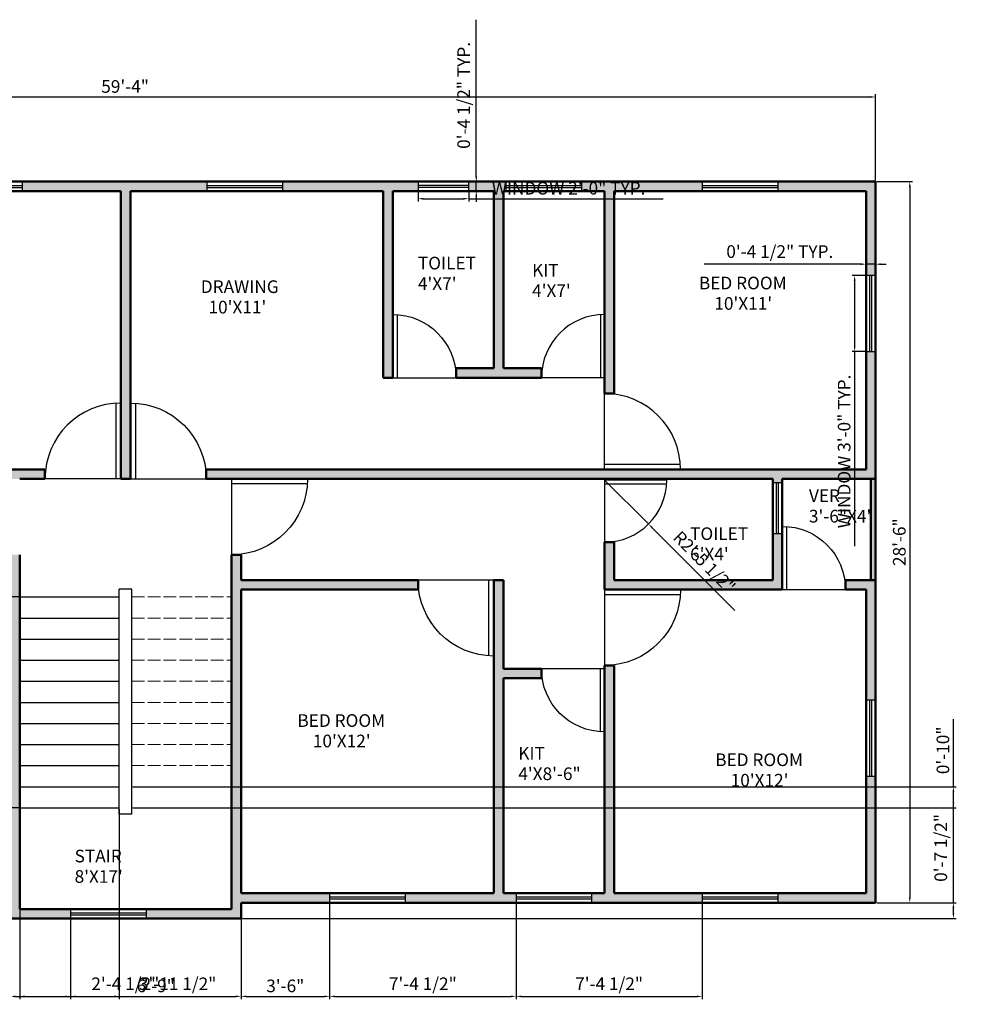
# Model space of a CAD drawing. Units: inches. Extents: x 1931 to 2735, y 1903 to 2370.
# Tile 2 of 2: x 2288 to 2735, y 1903 to 2370. Entities that reach past the tile are written whole.
import ezdxf

# ---------------------------------------------------------------- set-up
doc = ezdxf.new("R2010")
doc.units = ezdxf.units.IN
doc.header["$LTSCALE"] = 0.5
doc.linetypes.add('ACAD_ISO02W100', pattern=[15, 12, -3])
for name, color, linetype, lineweight in [('A-ANNO-DIMS', 93, 'Continuous', 18), ('A-AREA-IDEN', 93, 'Continuous', 25), ('A-FLOR-STRS', 231, 'Continuous', 25), ('A-FLOR-STRS-OVHD', 231, 'ACAD_ISO02W100', 18), ('DOORS', 121, 'Continuous', 25), ('WALLS', 231, 'Continuous', 50), ('WINDOWS', 200, 'Continuous', 25)]:
    doc.layers.add(name, color=color, linetype=linetype, lineweight=lineweight)
doc.layers.add('A-WALL-PATT', color=143, linetype='Continuous', lineweight=13, true_color=0x7aafdf)
doc.styles.get("Standard").update_dxf_attribs({"font": 'txt', "height": 6})
doc.dimstyles.new('ISO-25', dxfattribs={"dimtxt": 5, "dimasz": 2.5, "dimexe": 1.25, "dimexo": 0.625, "dimtad": 1, "dimlunit": 3, "dimtxsty": 'Standard', "dimcen": 2.5, "dimadec": 0, "dimazin": 0, "dimtfac": 1, "dimtmove": 0, "dimatfit": 3, "dimfxl": 1, "dimarcsym": 0})

# ---------------------------------------------------------------- blocks, each defined once
blk = doc.blocks.new('*D1')
at = {"layer": 'A-ANNO-DIMS', "color": 0, "lineweight": -2, "transparency": 16777216}
for p, q in [((1982.32, 2294.17), (1982.32, 2334.97)), ((1984.82, 2333.72), (2691.82, 2333.72)), ((2694.32, 2294.17), (2694.32, 2334.97))]:
    blk.add_line(p, q, dxfattribs=at)
at = {"layer": 'A-ANNO-DIMS', "color": 0, "lineweight": 100, "transparency": 16777216}
for points in [[(1984.82, 2334.14), (1984.82, 2333.3), (1982.32, 2333.72)], [(2691.82, 2334.14), (2691.82, 2333.3), (2694.32, 2333.72)]]:
    blk.add_solid(points, dxfattribs=at)
at = {"layer": 'Defpoints', "color": 0, "lineweight": 100, "transparency": 16777216}
for p in [(2694.32, 2333.72), (1982.32, 2293.55), (2694.32, 2293.55)]:
    blk.add_point(p, dxfattribs=at)
at = {"layer": 'A-ANNO-DIMS', "color": 0, "transparency": 16777216, "insert": (2338.32, 2337.92), "char_height": 6, "attachment_point": 5}
blk.add_mtext('59\'-4"', dxfattribs=at)
blk = doc.blocks.new('*D2')
at = {"layer": 'A-ANNO-DIMS', "color": 0, "lineweight": -2, "transparency": 16777216}
for p, q in [((2694.94, 2293.55), (2711.82, 2293.55)), ((2710.57, 2291.05), (2710.57, 1954.05)), ((2694.94, 1951.55), (2711.82, 1951.55))]:
    blk.add_line(p, q, dxfattribs=at)
at = {"layer": 'A-ANNO-DIMS', "color": 0, "lineweight": 100, "transparency": 16777216}
for points in [[(2710.16, 2291.05), (2710.99, 2291.05), (2710.57, 2293.55)], [(2710.16, 1954.05), (2710.99, 1954.05), (2710.57, 1951.55)]]:
    blk.add_solid(points, dxfattribs=at)
at = {"layer": 'Defpoints', "color": 0, "lineweight": 100, "transparency": 16777216}
for p in [(2694.32, 2293.55), (2694.32, 1951.55), (2710.57, 1951.55)]:
    blk.add_point(p, dxfattribs=at)
at = {"layer": 'A-ANNO-DIMS', "color": 0, "transparency": 16777216, "insert": (2706.38, 2122.55), "char_height": 6, "attachment_point": 5, "rotation": 90}
blk.add_mtext('28\'-6"', dxfattribs=at)
blk = doc.blocks.new('DOOR-SWING-36IN')
for p, q in [((0, 0), (0, 36)), ((35.92, 2.4), (0, 2.4)), ((36, 0), (0, 0))]:
    blk.add_line(p, q)
blk.add_arc((0, 0), 36, 0, 90)
blk = doc.blocks.new('DOOR-SWING-30IN')
for p, q in [((28, 29.93), (28, 0)), ((30, 30), (30, 0)), ((30, 0), (0, 0))]:
    blk.add_line(p, q)
blk.add_arc((30, 0), 30, 90, 180)
blk = doc.blocks.new('WINDOW-36IN')
for p, q in [((0, 36), (0, 0)), ((4.5, 36), (0, 36)), ((1.75, 36), (1.75, 0)), ((2.75, 36), (2.75, 0)), ((4.5, 0), (4.5, 36)), ((0, 0), (4.5, 0))]:
    blk.add_line(p, q)
blk = doc.blocks.new('WINDOW-24IN')
for p, q in [((24, 4.5), (0, 4.5)), ((0, 4.5), (0, 0)), ((24, 2.75), (0, 2.75)), ((24, 1.75), (0, 1.75)), ((0, 0), (24, 0)), ((24, 0), (24, 4.5))]:
    blk.add_line(p, q)
blk = doc.blocks.new('*D7')
at = {"layer": 'A-ANNO-DIMS', "color": 0, "lineweight": -2, "transparency": 16777216}
for p, q in [((2689.19, 2249), (2683.17, 2249)), ((2684.42, 2246.5), (2684.42, 2215.5)), ((2689.19, 2213), (2683.17, 2213)), ((2684.42, 2213), (2684.42, 2120.68))]:
    blk.add_line(p, q, dxfattribs=at)
at = {"layer": 'A-ANNO-DIMS', "color": 0, "lineweight": 100, "transparency": 16777216}
for points in [[(2684, 2246.5), (2684.83, 2246.5), (2684.42, 2249)], [(2684, 2215.5), (2684.83, 2215.5), (2684.42, 2213)]]:
    blk.add_solid(points, dxfattribs=at)
at = {"layer": 'Defpoints', "color": 0, "lineweight": 100, "transparency": 16777216}
for p in [(2689.82, 2249), (2684.42, 2213), (2689.82, 2213)]:
    blk.add_point(p, dxfattribs=at)
at = {"layer": 'A-ANNO-DIMS', "color": 0, "transparency": 16777216, "insert": (2680.22, 2165.59), "char_height": 6, "attachment_point": 5, "rotation": 90}
blk.add_mtext('WINDOW 3\'-0" TYP.', dxfattribs=at)
blk = doc.blocks.new('*D8')
at = {"layer": 'A-ANNO-DIMS', "color": 0, "lineweight": -2, "transparency": 16777216}
for p, q in [((2687.32, 2254.4), (2613, 2254.4)), ((2689.82, 2249.63), (2689.82, 2255.65)), ((2694.32, 2254.4), (2689.82, 2254.4)), ((2694.32, 2249.63), (2694.32, 2255.65)), ((2696.82, 2254.4), (2699.32, 2254.4))]:
    blk.add_line(p, q, dxfattribs=at)
at = {"layer": 'A-ANNO-DIMS', "color": 0, "lineweight": 100, "transparency": 16777216}
for points in [[(2687.32, 2254.82), (2687.32, 2253.99), (2689.82, 2254.4)], [(2696.82, 2254.82), (2696.82, 2253.99), (2694.32, 2254.4)]]:
    blk.add_solid(points, dxfattribs=at)
at = {"layer": 'Defpoints', "color": 0, "lineweight": 100, "transparency": 16777216}
for p in [(2689.82, 2254.4), (2689.82, 2249), (2694.32, 2249)]:
    blk.add_point(p, dxfattribs=at)
at = {"layer": 'A-ANNO-DIMS', "color": 0, "transparency": 16777216, "insert": (2648.91, 2259.6), "char_height": 6, "attachment_point": 5}
blk.add_mtext('0\'-4 1/2" TYP.', dxfattribs=at)
blk = doc.blocks.new('*D9')
at = {"layer": 'A-ANNO-DIMS', "color": 0, "lineweight": -2, "transparency": 16777216}
for p, q in [((2477.32, 2288.42), (2477.32, 2284.2)), ((2501.32, 2288.42), (2501.32, 2284.2)), ((2479.82, 2285.45), (2498.82, 2285.45)), ((2501.32, 2285.45), (2593.64, 2285.45))]:
    blk.add_line(p, q, dxfattribs=at)
at = {"layer": 'A-ANNO-DIMS', "color": 0, "lineweight": 100, "transparency": 16777216}
for points in [[(2479.82, 2285.86), (2479.82, 2285.03), (2477.32, 2285.45)], [(2498.82, 2285.86), (2498.82, 2285.03), (2501.32, 2285.45)]]:
    blk.add_solid(points, dxfattribs=at)
at = {"layer": 'Defpoints', "color": 0, "lineweight": 100, "transparency": 16777216}
for p in [(2477.32, 2289.05), (2501.32, 2289.05), (2501.32, 2285.45)]:
    blk.add_point(p, dxfattribs=at)
at = {"layer": 'A-ANNO-DIMS', "color": 0, "transparency": 16777216, "insert": (2548.73, 2289.64), "char_height": 6, "attachment_point": 5}
blk.add_mtext('WINDOW 2\'-0" TYP.', dxfattribs=at)
blk = doc.blocks.new('*D10')
at = {"layer": 'A-ANNO-DIMS', "color": 0, "lineweight": -2, "transparency": 16777216}
for p, q in [((2504.92, 2296.05), (2504.92, 2370.37)), ((2501.94, 2293.55), (2506.17, 2293.55)), ((2504.92, 2289.05), (2504.92, 2293.55)), ((2501.94, 2289.05), (2506.17, 2289.05)), ((2504.92, 2286.55), (2504.92, 2284.05))]:
    blk.add_line(p, q, dxfattribs=at)
at = {"layer": 'A-ANNO-DIMS', "color": 0, "lineweight": 100, "transparency": 16777216}
for points in [[(2504.5, 2296.05), (2505.33, 2296.05), (2504.92, 2293.55)], [(2504.5, 2286.55), (2505.33, 2286.55), (2504.92, 2289.05)]]:
    blk.add_solid(points, dxfattribs=at)
at = {"layer": 'Defpoints', "color": 0, "lineweight": 100, "transparency": 16777216}
for p in [(2501.32, 2293.55), (2504.92, 2293.55), (2501.32, 2289.05)]:
    blk.add_point(p, dxfattribs=at)
at = {"layer": 'A-ANNO-DIMS', "color": 0, "transparency": 16777216, "insert": (2499.72, 2334.46), "char_height": 6, "attachment_point": 5, "rotation": 90}
blk.add_mtext('0\'-4 1/2" TYP.', dxfattribs=at)
blk = doc.blocks.new('*D19')
at = {"layer": 'A-ANNO-DIMS', "color": 0, "lineweight": -2, "transparency": 16777216}
for p, q in [((2283.82, 1943.42), (2283.82, 1905.85)), ((2312.44, 1943.42), (2312.44, 1905.85)), ((2286.32, 1907.1), (2309.94, 1907.1)), ((2312.44, 1907.1), (2361.91, 1907.1))]:
    blk.add_line(p, q, dxfattribs=at)
at = {"layer": 'A-ANNO-DIMS', "color": 0, "lineweight": 100, "transparency": 16777216}
for points in [[(2286.32, 1907.51), (2286.32, 1906.68), (2283.82, 1907.1)], [(2309.94, 1907.51), (2309.94, 1906.68), (2312.44, 1907.1)]]:
    blk.add_solid(points, dxfattribs=at)
at = {"layer": 'Defpoints', "color": 0, "lineweight": 100, "transparency": 16777216}
for p in [(2283.82, 1944.05), (2312.44, 1944.05), (2312.44, 1907.1)]:
    blk.add_point(p, dxfattribs=at)
at = {"layer": 'A-ANNO-DIMS', "color": 0, "transparency": 16777216, "insert": (2338.42, 1912.29), "char_height": 6, "attachment_point": 5}
blk.add_mtext('2\'-4 1/2"', dxfattribs=at)
blk = doc.blocks.new('*D20')
at = {"layer": 'A-ANNO-DIMS', "color": 0, "lineweight": -2, "transparency": 16777216}
for p, q in [((2312.44, 1943.42), (2312.44, 1905.85)), ((2393.32, 1943.42), (2393.32, 1905.85)), ((2314.94, 1907.1), (2390.82, 1907.1))]:
    blk.add_line(p, q, dxfattribs=at)
at = {"layer": 'A-ANNO-DIMS', "color": 0, "lineweight": 100, "transparency": 16777216}
for points in [[(2314.94, 1907.51), (2314.94, 1906.68), (2312.44, 1907.1)], [(2390.82, 1907.51), (2390.82, 1906.68), (2393.32, 1907.1)]]:
    blk.add_solid(points, dxfattribs=at)
at = {"layer": 'Defpoints', "color": 0, "lineweight": 100, "transparency": 16777216}
for p in [(2312.44, 1944.05), (2393.32, 1944.05), (2393.32, 1907.1)]:
    blk.add_point(p, dxfattribs=at)
at = {"layer": 'A-ANNO-DIMS', "color": 0, "transparency": 16777216, "insert": (2352.88, 1911.29), "char_height": 6, "attachment_point": 5}
blk.add_mtext('6\'-9"', dxfattribs=at)
blk = doc.blocks.new('*D21')
at = {"layer": 'A-ANNO-DIMS', "color": 0, "lineweight": -2, "transparency": 16777216}
for p, q in [((2393.32, 1950.92), (2393.32, 1905.85)), ((2435.32, 1950.92), (2435.32, 1905.85)), ((2395.82, 1907.1), (2432.82, 1907.1))]:
    blk.add_line(p, q, dxfattribs=at)
at = {"layer": 'A-ANNO-DIMS', "color": 0, "lineweight": 100, "transparency": 16777216}
for points in [[(2395.82, 1907.51), (2395.82, 1906.68), (2393.32, 1907.1)], [(2432.82, 1907.51), (2432.82, 1906.68), (2435.32, 1907.1)]]:
    blk.add_solid(points, dxfattribs=at)
at = {"layer": 'Defpoints', "color": 0, "lineweight": 100, "transparency": 16777216}
for p in [(2393.32, 1951.55), (2435.32, 1951.55), (2435.32, 1907.1)]:
    blk.add_point(p, dxfattribs=at)
at = {"layer": 'A-ANNO-DIMS', "color": 0, "transparency": 16777216, "insert": (2414.32, 1911.29), "char_height": 6, "attachment_point": 5}
blk.add_mtext('3\'-6"', dxfattribs=at)
blk = doc.blocks.new('*D22')
at = {"layer": 'A-ANNO-DIMS', "color": 0, "lineweight": -2, "transparency": 16777216}
for p, q in [((2435.32, 1950.92), (2435.32, 1905.85)), ((2523.82, 1950.92), (2523.82, 1905.85)), ((2437.82, 1907.1), (2521.32, 1907.1))]:
    blk.add_line(p, q, dxfattribs=at)
at = {"layer": 'A-ANNO-DIMS', "color": 0, "lineweight": 100, "transparency": 16777216}
for points in [[(2437.82, 1907.51), (2437.82, 1906.68), (2435.32, 1907.1)], [(2521.32, 1907.51), (2521.32, 1906.68), (2523.82, 1907.1)]]:
    blk.add_solid(points, dxfattribs=at)
at = {"layer": 'Defpoints', "color": 0, "lineweight": 100, "transparency": 16777216}
for p in [(2435.32, 1951.55), (2523.82, 1951.55), (2523.82, 1907.1)]:
    blk.add_point(p, dxfattribs=at)
at = {"layer": 'A-ANNO-DIMS', "color": 0, "transparency": 16777216, "insert": (2479.57, 1912.29), "char_height": 6, "attachment_point": 5}
blk.add_mtext('7\'-4 1/2"', dxfattribs=at)
blk = doc.blocks.new('*D23')
at = {"layer": 'A-ANNO-DIMS', "color": 0, "lineweight": -2, "transparency": 16777216}
for p, q in [((2523.82, 1950.92), (2523.82, 1905.85)), ((2612.07, 1950.92), (2612.07, 1905.85)), ((2526.32, 1907.1), (2609.57, 1907.1))]:
    blk.add_line(p, q, dxfattribs=at)
at = {"layer": 'A-ANNO-DIMS', "color": 0, "lineweight": 100, "transparency": 16777216}
for points in [[(2526.32, 1907.51), (2526.32, 1906.68), (2523.82, 1907.1)], [(2609.57, 1907.51), (2609.57, 1906.68), (2612.07, 1907.1)]]:
    blk.add_solid(points, dxfattribs=at)
at = {"layer": 'Defpoints', "color": 0, "lineweight": 100, "transparency": 16777216}
for p in [(2523.82, 1951.55), (2612.07, 1951.55), (2612.07, 1907.1)]:
    blk.add_point(p, dxfattribs=at)
at = {"layer": 'A-ANNO-DIMS', "color": 0, "transparency": 16777216, "insert": (2567.94, 1912.29), "char_height": 6, "attachment_point": 5}
blk.add_mtext('7\'-4 1/2"', dxfattribs=at)
blk = doc.blocks.new('*D24')
at = {"layer": 'A-ANNO-DIMS', "color": 0, "lineweight": -2, "transparency": 16777216}
for p, q in [((2731.27, 1951.55), (2731.27, 2001.01)), ((2694.94, 1951.55), (2732.52, 1951.55)), ((2731.27, 1946.55), (2731.27, 1949.05)), ((2393.94, 1944.05), (2732.52, 1944.05))]:
    blk.add_line(p, q, dxfattribs=at)
at = {"layer": 'A-ANNO-DIMS', "color": 0, "lineweight": 100, "transparency": 16777216}
for points in [[(2730.85, 1949.05), (2731.68, 1949.05), (2731.27, 1951.55)], [(2730.85, 1946.55), (2731.68, 1946.55), (2731.27, 1944.05)]]:
    blk.add_solid(points, dxfattribs=at)
at = {"layer": 'Defpoints', "color": 0, "lineweight": 100, "transparency": 16777216}
for p in [(2694.32, 1951.55), (2731.27, 1951.55), (2393.32, 1944.05)]:
    blk.add_point(p, dxfattribs=at)
at = {"layer": 'A-ANNO-DIMS', "color": 0, "transparency": 16777216, "insert": (2726.07, 1977.53), "char_height": 6, "attachment_point": 5, "rotation": 90}
blk.add_mtext('0\'-7 1/2"', dxfattribs=at)
blk = doc.blocks.new('*D25')
at = {"layer": 'A-ANNO-DIMS', "color": 0, "lineweight": -2, "transparency": 16777216}
for p, q in [((2288.32, 1995.92), (2288.32, 1905.85)), ((2335.57, 1995.92), (2335.57, 1905.85)), ((2290.82, 1907.1), (2333.07, 1907.1)), ((2335.57, 1907.1), (2388.46, 1907.1))]:
    blk.add_line(p, q, dxfattribs=at)
at = {"layer": 'A-ANNO-DIMS', "color": 0, "lineweight": 100, "transparency": 16777216}
for points in [[(2290.82, 1907.51), (2290.82, 1906.68), (2288.32, 1907.1)], [(2333.07, 1907.51), (2333.07, 1906.68), (2335.57, 1907.1)]]:
    blk.add_solid(points, dxfattribs=at)
at = {"layer": 'Defpoints', "color": 0, "lineweight": 100, "transparency": 16777216}
for p in [(2288.32, 1996.55), (2335.57, 1996.55), (2335.57, 1907.1)]:
    blk.add_point(p, dxfattribs=at)
at = {"layer": 'A-ANNO-DIMS', "color": 0, "transparency": 16777216, "insert": (2363.26, 1912.29), "char_height": 6, "attachment_point": 5}
blk.add_mtext('3\'-11 1/2"', dxfattribs=at)
blk = doc.blocks.new('*D26')
at = {"layer": 'A-ANNO-DIMS', "color": 0, "lineweight": -2, "transparency": 16777216}
for p, q in [((2287.69, 2096.55), (1944.12, 2096.55)), ((1945.37, 1999.05), (1945.37, 2094.05)), ((2287.69, 1996.55), (1944.12, 1996.55))]:
    blk.add_line(p, q, dxfattribs=at)
at = {"layer": 'A-ANNO-DIMS', "color": 0, "lineweight": 100, "transparency": 16777216}
for points in [[(1944.95, 2094.05), (1945.78, 2094.05), (1945.37, 2096.55)], [(1944.95, 1999.05), (1945.78, 1999.05), (1945.37, 1996.55)]]:
    blk.add_solid(points, dxfattribs=at)
at = {"layer": 'Defpoints', "color": 0, "lineweight": 100, "transparency": 16777216}
for p in [(1945.37, 2096.55), (2288.32, 2096.55), (2288.32, 1996.55)]:
    blk.add_point(p, dxfattribs=at)
at = {"layer": 'A-ANNO-DIMS', "color": 0, "transparency": 16777216, "insert": (1941.17, 2046.55), "char_height": 6, "attachment_point": 5, "rotation": 90}
blk.add_mtext('8\'-4"', dxfattribs=at)
blk = doc.blocks.new('*D27')
at = {"layer": 'A-ANNO-DIMS', "color": 0, "lineweight": -2, "transparency": 16777216}
for p, q in [((2731.27, 2006.55), (2731.27, 2038.58)), ((2342.19, 2006.55), (2732.52, 2006.55)), ((2731.27, 1999.05), (2731.27, 2004.05)), ((2342.19, 1996.55), (2732.52, 1996.55))]:
    blk.add_line(p, q, dxfattribs=at)
at = {"layer": 'A-ANNO-DIMS', "color": 0, "lineweight": 100, "transparency": 16777216}
for points in [[(2730.85, 2004.05), (2731.68, 2004.05), (2731.27, 2006.55)], [(2730.85, 1999.05), (2731.68, 1999.05), (2731.27, 1996.55)]]:
    blk.add_solid(points, dxfattribs=at)
at = {"layer": 'Defpoints', "color": 0, "lineweight": 100, "transparency": 16777216}
for p in [(2341.57, 2006.55), (2731.27, 2006.55), (2341.57, 1996.55)]:
    blk.add_point(p, dxfattribs=at)
at = {"layer": 'A-ANNO-DIMS', "color": 0, "transparency": 16777216, "insert": (2727.07, 2023.81), "char_height": 6, "attachment_point": 5, "rotation": 90}
blk.add_mtext('0\'-10"', dxfattribs=at)
blk = doc.blocks.new('*D30')
at = {"layer": 'A-ANNO-DIMS', "color": 0, "lineweight": -2, "transparency": 16777216}
for p, q in [((2565.82, 2151.98), (2586.63, 2131.17)), ((2627.62, 2090.18), (2588.4, 2129.4))]:
    blk.add_line(p, q, dxfattribs=at)
at = {"layer": 'A-ANNO-DIMS', "color": 0, "lineweight": 100, "transparency": 16777216}
blk.add_solid([(2588.69, 2129.69), (2588.1, 2129.1), (2586.63, 2131.17)], dxfattribs=at)
at = {"layer": 'Defpoints', "color": 0, "lineweight": 100, "transparency": 16777216}
for p in [(2565.82, 2151.98), (2586.63, 2131.17)]:
    blk.add_point(p, dxfattribs=at)
at = {"layer": 'A-ANNO-DIMS', "color": 0, "transparency": 16777216, "insert": (2612.57, 2112.58), "char_height": 6, "attachment_point": 5, "rotation": 315.0004}
blk.add_mtext('R2\'-5 1/2"', dxfattribs=at)

msp = doc.modelspace()

# ---------------------------------------------------------------- hatches: boundary and pattern name
at = {"layer": 'A-WALL-PATT'}
h = msp.add_hatch(color=256, dxfattribs=at)
h.dxf.hatch_style = 1
h.paths.add_polyline_path([(2028.817, 2293.545), (1982.317, 2293.545), (1982.317, 2249.002), (1986.817, 2249.002), (1986.817, 2289.045), (2028.817, 2289.045)])
h.paths.add_polyline_path([(2113.054, 2293.545), (2064.817, 2293.545), (2064.817, 2289.045), (2106.817, 2289.045), (2106.817, 2193.045), (2111.317, 2193.045), (2111.317, 2200.545), (2111.317, 2230.545), (2111.317, 2289.045), (2113.054, 2289.045)])
h.paths.add_polyline_path([(2175.817, 2293.545), (2149.054, 2293.545), (2149.054, 2289.045), (2159.317, 2289.045), (2159.317, 2205.045), (2141.317, 2205.045), (2141.317, 2200.545), (2181.817, 2200.545), (2181.817, 2205.045), (2163.817, 2205.045), (2163.817, 2289.045), (2175.817, 2289.045)])
h.paths.add_polyline_path([(2253.691, 2293.545), (2199.817, 2293.545), (2199.817, 2289.045), (2211.817, 2289.045), (2211.817, 2200.545), (2216.317, 2200.545), (2216.317, 2289.045), (2253.691, 2289.045)])
h.paths.add_polyline_path([(2377.162, 2293.545), (2289.691, 2293.545), (2289.691, 2289.045), (2336.317, 2289.045), (2336.317, 2152.545), (2340.817, 2152.545), (2340.817, 2188.545), (2340.817, 2289.045), (2377.162, 2289.045)])
h.paths.add_polyline_path([(2477.317, 2293.545), (2413.162, 2293.545), (2413.162, 2289.045), (2460.817, 2289.045), (2460.817, 2200.545), (2465.317, 2200.545), (2465.317, 2230.545), (2465.317, 2289.045), (2477.317, 2289.045)])
h.paths.add_polyline_path([(2518.935, 2293.545), (2501.317, 2293.545), (2501.317, 2289.045), (2513.317, 2289.045), (2513.317, 2205.045), (2495.317, 2205.045), (2495.317, 2200.545), (2535.817, 2200.545), (2535.817, 2205.045), (2517.817, 2205.045), (2517.817, 2289.045), (2518.935, 2289.045)])
h.paths.add_polyline_path([(2612.067, 2293.545), (2554.935, 2293.545), (2554.935, 2289.045), (2565.817, 2289.045), (2565.817, 2200.545), (2565.817, 2193.045), (2570.317, 2193.045), (2570.317, 2289.045), (2612.067, 2289.045)])
h.paths.add_polyline_path([(2694.317, 2293.545), (2648.067, 2293.545), (2648.067, 2289.045), (2689.817, 2289.045), (2689.817, 2249.002), (2694.317, 2249.002)])
h.paths.add_polyline_path([(2694.317, 2213.002), (2689.817, 2213.002), (2689.817, 2157.045), (2565.817, 2157.045), (2376.817, 2157.045), (2376.817, 2152.545), (2388.817, 2152.545), (2424.817, 2152.545), (2565.817, 2152.545), (2645.567, 2152.545), (2645.567, 2150.653), (2650.067, 2150.653), (2650.067, 2152.545), (2694.317, 2152.545)])
h.paths.add_polyline_path([(2694.317, 2152.545), (2692.067, 2152.545), (2692.067, 2104.545), (2694.317, 2104.545)])
h.paths.add_polyline_path([(2694.317, 2104.545), (2680.067, 2104.545), (2680.067, 2100.045), (2689.817, 2100.045), (2689.817, 2047.537), (2694.317, 2047.537)])
h.paths.add_polyline_path([(2650.067, 2126.653), (2645.567, 2126.653), (2645.567, 2104.545), (2570.317, 2104.545), (2570.317, 2122.545), (2565.817, 2122.545), (2565.817, 2100.045), (2601.817, 2100.045), (2650.067, 2100.045)])
h.paths.add_polyline_path([(2570.317, 2064.045), (2565.817, 2064.045), (2565.817, 2062.545), (2565.817, 2032.545), (2565.817, 1956.045), (2559.817, 1956.045), (2559.817, 1951.545), (2612.067, 1951.545), (2612.067, 1956.045), (2570.317, 1956.045)])
h.paths.add_polyline_path([(2694.317, 2011.537), (2689.817, 2011.537), (2689.817, 1956.045), (2648.067, 1956.045), (2648.067, 1951.545), (2694.317, 1951.545)])
h.paths.add_polyline_path([(2435.317, 1956.045), (2393.317, 1956.045), (2393.317, 2100.045), (2477.317, 2100.045), (2477.317, 2104.545), (2393.317, 2104.545), (2393.317, 2116.545), (2388.817, 2116.545), (2388.817, 1948.545), (2348.443, 1948.545), (2348.443, 1944.045), (2393.317, 1944.045), (2393.317, 1951.545), (2435.317, 1951.545)])
h.paths.add_polyline_path([(2523.817, 1956.045), (2517.817, 1956.045), (2517.817, 2058.045), (2535.817, 2058.045), (2535.817, 2062.545), (2517.817, 2062.545), (2517.817, 2104.545), (2513.317, 2104.545), (2513.317, 2068.545), (2513.317, 1956.045), (2471.317, 1956.045), (2471.317, 1951.545), (2523.817, 1951.545)])
h.paths.add_polyline_path([(2288.317, 2116.545), (2283.817, 2116.545), (2283.817, 2104.545), (2199.817, 2104.545), (2199.817, 2100.045), (2283.817, 2100.045), (2283.817, 1956.045), (2237.745, 1956.045), (2237.745, 1951.545), (2283.817, 1951.545), (2283.817, 1944.045), (2312.443, 1944.045), (2312.443, 1948.545), (2288.317, 1948.545)])
h.paths.add_polyline_path([(2163.817, 2104.545), (2159.317, 2104.545), (2159.317, 2062.545), (2111.317, 2062.545), (2111.317, 2064.045), (2106.817, 2064.045), (2106.817, 1956.045), (2064.817, 1956.045), (2064.817, 1951.545), (2117.317, 1951.545), (2117.317, 1956.045), (2111.317, 1956.045), (2111.317, 2058.045), (2159.317, 2058.045), (2159.317, 1956.045), (2153.317, 1956.045), (2153.317, 1951.545), (2201.745, 1951.545), (2201.745, 1956.045), (2163.817, 1956.045)])
h.paths.add_polyline_path([(2031.067, 2127.762), (2026.567, 2127.762), (2026.567, 2100.045), (2111.317, 2100.045), (2111.317, 2122.545), (2106.817, 2122.545), (2106.817, 2104.545), (2031.067, 2104.545)])
h.paths.add_polyline_path([(1996.567, 2104.545), (1982.317, 2104.545), (1982.317, 2046.045), (1986.817, 2046.045), (1986.817, 2100.045), (1996.567, 2100.045)])
h.paths.add_polyline_path([(1986.817, 2010.045), (1982.317, 2010.045), (1982.317, 1951.545), (2028.817, 1951.545), (2028.817, 1956.045), (1986.817, 1956.045)])
h.paths.add_polyline_path([(1984.567, 2152.545), (1982.317, 2152.545), (1982.317, 2104.545), (1984.567, 2104.545)])
h.paths.add_polyline_path([(1986.817, 2213.002), (1982.317, 2213.002), (1982.317, 2152.545), (1984.567, 2152.545), (2026.567, 2152.545), (2026.567, 2151.762), (2031.067, 2151.762), (2031.067, 2152.545), (2111.317, 2152.545), (2288.317, 2152.545), (2300.317, 2152.545), (2300.317, 2157.045), (2111.317, 2157.045), (2075.317, 2157.045), (1986.817, 2157.045)])

# ---------------------------------------------------------------- linework, layer by layer
at = {"layer": 'A-FLOR-STRS'}
for p, q in [((2335.567, 1993.494), (2335.567, 2100.31)), ((2341.567, 2100.31), (2335.567, 2100.31)), ((2341.567, 1993.494), (2341.567, 2100.31)), ((2288.317, 2096.545), (2335.567, 2096.545)), ((2288.317, 2086.545), (2335.567, 2086.545)), ((2288.317, 2076.545), (2335.567, 2076.545)), ((2288.317, 2066.545), (2335.567, 2066.545)), ((2288.317, 2056.545), (2335.567, 2056.545)), ((2288.317, 2046.545), (2335.567, 2046.545)), ((2288.317, 2036.545), (2335.567, 2036.545)), ((2288.317, 2026.545), (2335.567, 2026.545)), ((2288.317, 2016.545), (2335.567, 2016.545)), ((2288.317, 2006.545), (2335.567, 2006.545)), ((2288.317, 1996.545), (2335.567, 1996.545)), ((2341.567, 1993.494), (2335.567, 1993.494))]:
    msp.add_line(p, q, dxfattribs=at)
msp.add_lwpolyline([(2311.942, 2106.358, 0, 0, 0), (2311.942, 1981.649, 0, 0, 0), (2365.192, 1981.649, 0, 0, 0), (2365.192, 2058.853, 6, 0, 0), (2365.192, 2066.545, 0, 0, 0)], format="xyseb", dxfattribs=at)
at = {"layer": 'A-FLOR-STRS-OVHD'}
for p, q in [((2341.567, 2096.545), (2388.817, 2096.545)), ((2341.567, 2086.545), (2388.817, 2086.545)), ((2341.567, 2076.545), (2388.817, 2076.545)), ((2341.567, 2066.545), (2388.817, 2066.545)), ((2341.567, 2056.545), (2388.817, 2056.545)), ((2341.567, 2046.545), (2388.817, 2046.545)), ((2341.567, 2036.545), (2388.817, 2036.545)), ((2341.567, 2026.545), (2388.817, 2026.545)), ((2341.567, 2016.545), (2388.817, 2016.545)), ((2341.567, 2006.545), (2388.817, 2006.545)), ((2341.567, 1996.545), (2388.817, 1996.545))]:
    msp.add_line(p, q, dxfattribs=at)
at = {"layer": 'DOORS'}
for p, q in [((2595.251, 2151.978), (2565.817, 2151.978)), ((2565.817, 2151.978), (2565.817, 2122.545)), ((2595.185, 2150.016), (2565.817, 2150.016))]:
    msp.add_line(p, q, dxfattribs=at)
msp.add_arc((2565.817, 2151.978), 29.433, 270, 0, dxfattribs=at)
at = {"layer": 'WALLS'}
for p, q in [((1982.317, 2293.545), (2694.317, 2293.545)), ((2694.317, 2293.545), (2694.317, 1951.545)), ((2216.317, 2289.045), (2336.317, 2289.045)), ((2336.317, 2152.545), (2336.317, 2289.045)), ((2340.817, 2152.545), (2340.817, 2289.045)), ((2340.817, 2289.045), (2460.817, 2289.045)), ((2460.817, 2200.545), (2460.817, 2289.045)), ((2465.317, 2200.545), (2465.317, 2289.045)), ((2465.317, 2289.045), (2513.317, 2289.045)), ((2513.317, 2205.045), (2513.317, 2289.045)), ((2513.317, 2205.045), (2513.317, 2289.045)), ((2517.817, 2205.045), (2517.817, 2289.045)), ((2517.817, 2205.045), (2517.817, 2289.045)), ((2517.817, 2289.045), (2565.817, 2289.045)), ((2565.817, 2200.545), (2565.817, 2289.045)), ((2570.317, 2193.045), (2570.317, 2289.045)), ((2570.317, 2289.045), (2689.817, 2289.045)), ((2689.817, 2289.045), (2689.817, 2157.045)), ((2495.317, 2205.045), (2513.317, 2205.045)), ((2495.317, 2200.545), (2495.317, 2205.045)), ((2517.817, 2205.045), (2535.817, 2205.045)), ((2535.817, 2200.545), (2535.817, 2205.045)), ((2460.817, 2200.545), (2465.317, 2200.545)), ((2495.317, 2200.545), (2535.817, 2200.545)), ((2565.817, 2193.045), (2565.817, 2200.545)), ((2565.817, 2193.045), (2570.317, 2193.045)), ((2111.317, 2157.045), (2300.317, 2157.045)), ((2300.317, 2152.545), (2300.317, 2157.045)), ((2376.817, 2157.045), (2565.817, 2157.045)), ((2376.817, 2152.545), (2376.817, 2157.045)), ((2565.817, 2157.045), (2689.817, 2157.045)), ((2288.317, 2152.545), (2300.317, 2152.545)), ((2336.317, 2152.545), (2340.817, 2152.545)), ((2376.817, 2152.545), (2388.817, 2152.545)), ((2388.817, 2152.545), (2565.817, 2152.545)), ((2565.817, 2152.545), (2645.567, 2152.545)), ((2645.567, 2104.545), (2645.567, 2152.545)), ((2650.067, 2100.045), (2650.067, 2152.545)), ((2650.067, 2152.545), (2694.317, 2152.545)), ((2692.067, 2104.545), (2692.067, 2152.545)), ((2565.817, 2100.045), (2565.817, 2122.545)), ((2565.817, 2122.545), (2570.317, 2122.545)), ((2570.317, 2104.545), (2570.317, 2122.545)), ((2288.317, 1948.545), (2288.317, 2116.545)), ((2388.817, 1948.545), (2388.817, 2116.545)), ((2388.817, 2116.545), (2393.317, 2116.545)), ((2393.317, 2104.545), (2393.317, 2116.545)), ((2393.317, 2104.545), (2477.317, 2104.545)), ((2477.317, 2100.045), (2477.317, 2104.545)), ((2513.317, 1956.045), (2513.317, 2104.545)), ((2513.317, 2104.545), (2517.817, 2104.545)), ((2517.817, 2062.545), (2517.817, 2104.545)), ((2570.317, 2104.545), (2645.567, 2104.545)), ((2680.067, 2104.545), (2694.317, 2104.545)), ((2680.067, 2100.045), (2680.067, 2104.545)), ((2393.317, 2100.045), (2477.317, 2100.045)), ((2393.317, 1956.045), (2393.317, 2100.045)), ((2565.817, 2100.045), (2650.067, 2100.045)), ((2680.067, 2100.045), (2689.817, 2100.045)), ((2689.817, 2100.045), (2689.817, 1956.045)), ((2535.817, 2062.545), (2517.817, 2062.545)), ((2535.817, 2058.045), (2535.817, 2062.545)), ((2565.817, 2062.545), (2565.817, 2064.045)), ((2565.817, 2064.045), (2570.317, 2064.045)), ((2565.817, 1956.045), (2565.817, 2062.545)), ((2570.317, 1956.045), (2570.317, 2064.045)), ((2535.817, 2058.045), (2517.817, 2058.045)), ((2517.817, 1956.045), (2517.817, 2058.045)), ((2513.317, 1956.045), (2393.317, 1956.045)), ((2565.817, 1956.045), (2517.817, 1956.045)), ((2689.817, 1956.045), (2570.317, 1956.045)), ((2288.317, 1948.545), (2388.817, 1948.545)), ((2694.317, 1951.545), (2393.317, 1951.545)), ((2393.317, 1944.045), (2393.317, 1951.545)), ((2283.817, 1944.045), (2393.317, 1944.045))]:
    msp.add_line(p, q, dxfattribs=at)

# ---------------------------------------------------------------- block references
at = {"layer": 'DOORS', "extrusion": (0, 0, -1), "zscale": -1}
for p in [(-2495.318, 2200.545), (-2680.068, 2100.045)]:
    msp.add_blockref('DOOR-SWING-30IN', p, dxfattribs=at)
at = {"layer": 'DOORS'}
for name, p in [('DOOR-SWING-30IN', (2535.817, 2200.545)), ('DOOR-SWING-36IN', (2565.817, 2157.045))]:
    msp.add_blockref(name, p, dxfattribs=at)
at = {"layer": 'DOORS', "rotation": 90.0000000000022}
msp.add_blockref('DOOR-SWING-36IN', (2336.318, 2152.545), dxfattribs=at)
at = {"layer": 'DOORS', "extrusion": (0, 0, -1), "zscale": -1}
for name, p, rotation in [('DOOR-SWING-36IN', (-2340.817, 2152.545), 90.00000000000017), ('DOOR-SWING-36IN', (-2388.817, 2152.545), 180), ('DOOR-SWING-36IN', (-2513.318, 2104.546), 269.9999999999998), ('DOOR-SWING-36IN', (-2565.817, 2100.045), 180), ('DOOR-SWING-30IN', (-2535.817, 2062.545), 180)]:
    msp.add_blockref(name, p, dxfattribs=dict(at, rotation=rotation))
at = {"layer": 'WINDOWS'}
for name, p, rotation in [('WINDOW-36IN', (2289.691, 2289.045), 90.00000000000072), ('WINDOW-36IN', (2413.162, 2289.045), 90.00000000000072), ('WINDOW-36IN', (2554.936, 2289.045), 90.00000000000018), ('WINDOW-36IN', (2648.068, 2289.045), 90.00000000000072), ('WINDOW-36IN', (2694.318, 2249.002), 180), ('WINDOW-24IN', (2645.567, 2150.654), 270.0000000000038), ('WINDOW-36IN', (2694.318, 2047.537), 180), ('WINDOW-36IN', (2471.318, 1951.545), 90.00000000000144), ('WINDOW-36IN', (2559.818, 1951.545), 90.00000000000144), ('WINDOW-36IN', (2648.068, 1951.545), 90.00000000000144), ('WINDOW-36IN', (2348.443, 1944.045), 90.00000000000144)]:
    msp.add_blockref(name, p, dxfattribs=dict(at, rotation=rotation))
msp.add_blockref('WINDOW-24IN', (2477.317, 2289.045), dxfattribs=at)

# ---------------------------------------------------------------- texts
at = {"layer": 'A-AREA-IDEN'}
for s, p in [('TOILET', (2477.229, 2251.926)), ('KIT', (2531.399, 2248.543)), ('DRAWING', (2374.223, 2240.729)), ("4'X7'", (2477.229, 2242.227)), ('BED ROOM', (2610.52, 2242.464)), ("4'X7'", (2531.399, 2238.844)), ("  10'X11'", (2374.223, 2231.031)), ("    10'X11'", (2610.52, 2232.765)), ('VER', (2662.735, 2141.57)), ('3\'-6"X4\'', (2662.735, 2131.871)), ('TOILET', (2606.347, 2123.585)), ("6'X4'", (2606.347, 2113.887)), ('BED ROOM', (2420.057, 2034.942)), ("    10'X12'", (2420.057, 2025.243)), ('KIT ', (2524.864, 2019.397)), ('BED ROOM', (2618.271, 2016.329)), ('4\'X8\'-6"', (2524.864, 2009.699)), ("    10'X12'", (2618.271, 2006.63)), ('STAIR', (2314.378, 1970.667)), ("8'X17'", (2314.378, 1960.969))]:
    msp.add_text(s, height=6, dxfattribs=at).set_placement(p)

# ---------------------------------------------------------------- dimensions: what is measured, and where the dimension line sits
at = {"layer": 'A-ANNO-DIMS'}
for base, p1, p2, angle, text, picture, middle in [((2504.917, 2293.545), (2501.317, 2289.045), (2501.317, 2293.545), 90, '<> TYP.', '*D10', (2499.721, 2334.456)), ((2689.817, 2254.402), (2694.317, 2249.002), (2689.817, 2249.002), 180, '<> TYP.', '*D8', (2648.907, 2259.599)), ((2684.417, 2213.002), (2689.817, 2249.002), (2689.817, 2213.002), 270, 'WINDOW <> TYP.', '*D7', (2680.221, 2165.592))]:
    dim = msp.add_linear_dim(base=base, p1=p1, p2=p2, angle=angle, text=text, dimstyle='ISO-25', override={"dimdec": 1, "dimlfac": 1, "dimrnd": 0, "dimzin": 1, "dimdsep": 46, "dimlunit": 4, "dimfrac": 2}, dxfattribs=at)
    dim.commit()
    dim.dimension.update_dxf_attribs({"geometry": picture, "text_midpoint": middle})
for base, p1, p2, override, picture, middle in [((2694.317, 2333.721), (1982.317, 2293.545), (2694.317, 2293.545), {"dimclrd": 0, "dimclre": 0, "dimclrt": 0}, '*D1', (2338.317, 2337.918)), ((2335.567423, 1907.09517), (2288.317423, 1996.54517), (2335.567423, 1996.54517), {"dimdec": 1, "dimlfac": 1, "dimrnd": 0, "dimzin": 1, "dimdsep": 46, "dimlunit": 4, "dimfrac": 2}, '*D25', (2363.263851571, 1912.291598571)), ((2435.317, 1907.095), (2393.317, 1951.545), (2435.317, 1951.545), {"dimdec": 1, "dimlfac": 1, "dimrnd": 0, "dimzin": 1, "dimdsep": 46, "dimlunit": 4, "dimfrac": 2}, '*D21', (2414.317, 1911.292)), ((2523.817, 1907.095), (2435.317, 1951.545), (2523.817, 1951.545), {"dimdec": 1, "dimlfac": 1, "dimrnd": 0, "dimzin": 1, "dimdsep": 46, "dimlunit": 4, "dimfrac": 2}, '*D22', (2479.567, 1912.292)), ((2612.067423, 1907.09517), (2523.817423, 1951.54517), (2612.067423, 1951.54517), {"dimdec": 1, "dimlfac": 1, "dimrnd": 0, "dimzin": 1, "dimdsep": 46, "dimlunit": 4, "dimfrac": 2}, '*D23', (2567.942423, 1912.291598571)), ((2312.443, 1907.095), (2283.817, 1944.045), (2312.443, 1944.045), {"dimdec": 1, "dimlfac": 1, "dimrnd": 0, "dimzin": 1, "dimdsep": 46, "dimlunit": 4, "dimfrac": 2}, '*D19', (2338.425, 1912.292)), ((2393.317, 1907.095), (2312.443, 1944.045), (2393.317, 1944.045), {"dimdec": 1, "dimlfac": 1, "dimrnd": 0, "dimzin": 1, "dimdsep": 46, "dimlunit": 4, "dimfrac": 2}, '*D20', (2352.88, 1911.292))]:
    dim = msp.add_linear_dim(base=base, p1=p1, p2=p2, dimstyle='ISO-25', override=override, dxfattribs=at)
    dim.commit()
    dim.dimension.update_dxf_attribs({"geometry": picture, "text_midpoint": middle})
dim = msp.add_linear_dim(base=(2501.317, 2285.445), p1=(2477.317, 2289.045), p2=(2501.317, 2289.045), text='WINDOW <> TYP.', dimstyle='ISO-25', override={"dimdec": 1, "dimlfac": 1, "dimrnd": 0, "dimzin": 1, "dimdsep": 46, "dimlunit": 4, "dimfrac": 2}, dxfattribs=at)
dim.commit()
dim.dimension.update_dxf_attribs({"geometry": '*D9', "text_midpoint": (2548.728, 2289.642)})
for base, p1, p2, override, picture, middle in [((2710.573, 1951.545), (2694.317, 2293.545), (2694.317, 1951.545), {"dimclrd": 0, "dimclre": 0, "dimclrt": 0}, '*D2', (2706.377, 2122.545)), ((1945.367, 2096.545), (2288.317, 1996.545), (2288.317, 2096.545), {"dimdec": 1, "dimlfac": 1, "dimrnd": 0, "dimzin": 1, "dimdsep": 46, "dimlunit": 4, "dimfrac": 2}, '*D26', (1941.171, 2046.545)), ((2731.267, 2006.545), (2341.567, 1996.545), (2341.567, 2006.545), {"dimdec": 1, "dimlfac": 1, "dimrnd": 0, "dimzin": 1, "dimdsep": 46, "dimlunit": 4, "dimfrac": 2}, '*D27', (2727.071, 2023.813)), ((2731.267, 1951.545), (2393.317, 1944.045), (2694.317, 1951.545), {"dimdec": 1, "dimlfac": 1, "dimrnd": 0, "dimzin": 1, "dimdsep": 46, "dimlunit": 4, "dimfrac": 2}, '*D24', (2726.071, 1977.527))]:
    dim = msp.add_linear_dim(base=base, p1=p1, p2=p2, angle=90, dimstyle='ISO-25', override=override, dxfattribs=at)
    dim.commit()
    dim.dimension.update_dxf_attribs({"geometry": picture, "text_midpoint": middle})
dim = msp.add_radius_dim(center=(2565.817, 2151.978), mpoint=(2586.63, 2131.166), dimstyle='ISO-25', override={"dimdec": 1, "dimlfac": 1, "dimrnd": 0, "dimzin": 1, "dimdsep": 46, "dimlunit": 4, "dimfrac": 2}, dxfattribs=at)
dim.commit()
dim.dimension.update_dxf_attribs({"geometry": '*D30', "text_midpoint": (2612.566, 2112.579)})

doc.saveas('drawing.dxf')
